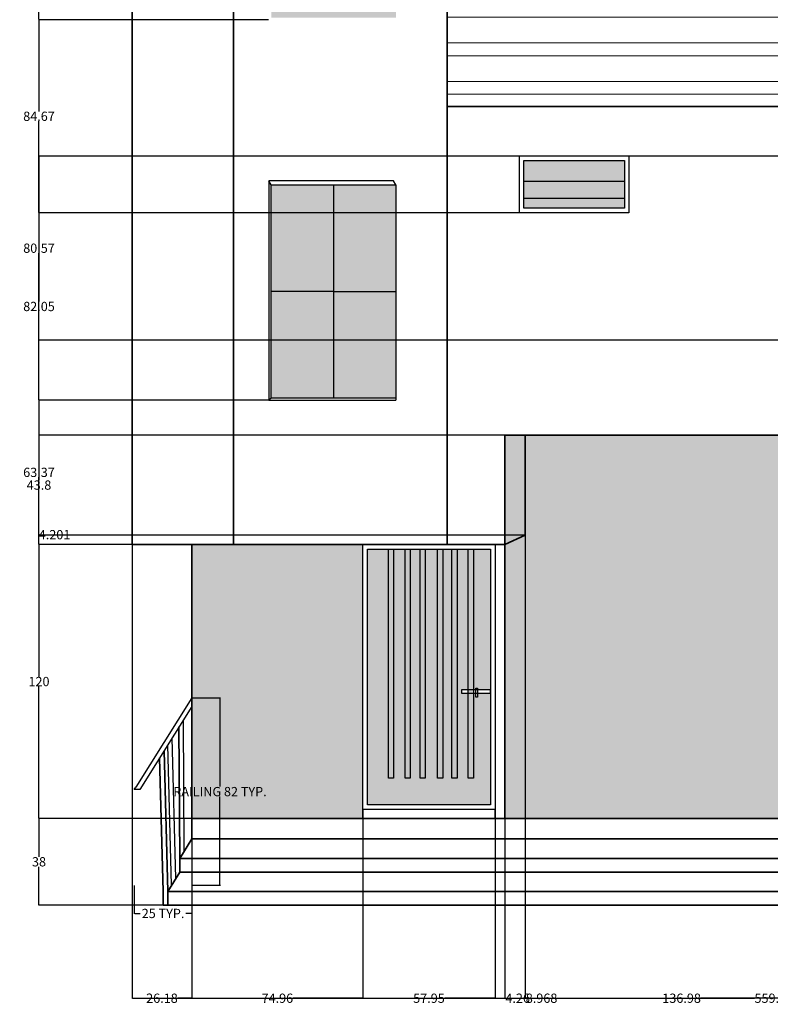
# Model space of a CAD drawing. Units: inches. Extents: x -35 to 623, y 74 to 964.
# Tile 1 of 3: x -35 to 294, y 74 to 505. Entities that reach past the tile are written whole.
import ezdxf

# ---------------------------------------------------------------- set-up
doc = ezdxf.new("R2010")
doc.units = ezdxf.units.IN
doc.header["$MEASUREMENT"] = 0
for name, color, linetype, lineweight in [('A-ANNO-DIMS', 2, 'Continuous', 18), ('A-DOOR', 3, 'Continuous', 25), ('A-ELEV', 7, 'Continuous', 35), ('A-ELEV-PATT', 8, 'Continuous', 13), ('A-FLOR-STRS', 7, 'Continuous', 25), ('A-GLAZ', 4, 'Continuous', 25)]:
    doc.layers.add(name, color=color, linetype=linetype, lineweight=lineweight)
doc.styles.get("Standard").update_dxf_attribs({"font": 'arial.ttf'})
doc.dimstyles.get("Standard").update_dxf_attribs({"dimtxt": 4.0625, "dimasz": 0.18, "dimexe": 0.18, "dimexo": 0.0625, "dimgap": 0.09, "dimtad": 0, "dimtih": 1, "dimtoh": 1, "dimdec": 4, "dimzin": 0, "dimdsep": 46, "dimlunit": 4, "dimtxsty": 'Standard', "dimcen": 0.09, "dimadec": 0, "dimazin": 0, "dimtfac": 1, "dimtdec": 4, "dimtofl": 0, "dimtmove": 0, "dimatfit": 3, "dimfxl": 1, "dimtolj": 1, "dimtzin": 0, "dimarcsym": 0})

# ---------------------------------------------------------------- blocks, each defined once
blk = doc.blocks.new('WIN-TALL-2X2')
for p, q in [((1.05, 94.39), (0, 96.09)), ((0, 96.09), (0, 0)), ((54.58, 96.06), (0, 96.06)), ((55.68, 94.39), (54.58, 96.06)), ((28.36, 94.39), (28.36, 0.82)), ((1.05, 0.82), (0, 0)), ((55.68, 0.82), (55.68, 0)), ((0, 0), (55.68, 0))]:
    blk.add_line(p, q)
blk.add_lwpolyline([(1.05, 94.39), (55.68, 94.39), (55.68, 0.82), (1.05, 0.82)], close=True)
blk = doc.blocks.new('VENT-FRAME')
for points in [[(0, 25.02), (48.03, 25.02), (48.03, 0), (0, 0)], [(2, 23.02), (46.03, 23.02), (46.03, 2), (2, 2)]]:
    blk.add_lwpolyline(points, close=True)
blk = doc.blocks.new('STAIR-RAIL')
for p, q in [((25.22, 82.16), (0.67, 43)), ((25.22, 78.4), (2.36, 41.93)), ((21.93, 15.01), (21.56, 72.56)), ((16.35, 0), (14.7, 61.62)), ((18.27, 3.03), (16.62, 64.68)), ((0, 41.93), (0.67, 43)), ((2.36, 41.93), (0, 41.93))]:
    blk.add_line(p, q)
blk = doc.blocks.new('*D11')
at = {"layer": 'A-ANNO-DIMS', "color": 0, "lineweight": -2, "transparency": 16777216}
for p, q in [((40.51, 207.97), (52.95, 207.97)), ((52.77, 207.79), (52.77, 169.08)), ((52.77, 125.99), (52.77, 164.7)), ((40.51, 125.81), (52.95, 125.81))]:
    blk.add_line(p, q, dxfattribs=at)
at = {"layer": 'A-ANNO-DIMS', "color": 0, "transparency": 16777216}
for points in [[(52.74, 207.79), (52.8, 207.79), (52.77, 207.97)], [(52.74, 125.99), (52.8, 125.99), (52.77, 125.81)]]:
    blk.add_solid(points, dxfattribs=at)
at = {"layer": 'Defpoints', "color": 0, "transparency": 16777216}
for p in [(40.44, 207.97), (52.77, 207.97), (40.44, 125.81)]:
    blk.add_point(p, dxfattribs=at)
at = {"layer": 'A-ANNO-DIMS', "color": 0, "transparency": 16777216, "insert": (52.77, 166.89), "char_height": 4.0625, "attachment_point": 5}
blk.add_mtext('\\A1;RAILING 82 TYP.', dxfattribs=at)
blk = doc.blocks.new('*D12')
at = {"layer": 'A-ANNO-DIMS', "color": 0, "lineweight": -2, "transparency": 16777216}
for p, q in [((15.22, 125.75), (15.22, 113.31)), ((40.44, 125.75), (40.44, 113.31)), ((15.4, 113.49), (17.82, 113.49)), ((40.26, 113.49), (37.84, 113.49))]:
    blk.add_line(p, q, dxfattribs=at)
at = {"layer": 'A-ANNO-DIMS', "color": 0, "transparency": 16777216}
for points in [[(15.4, 113.52), (15.4, 113.46), (15.22, 113.49)], [(40.26, 113.52), (40.26, 113.46), (40.44, 113.49)]]:
    blk.add_solid(points, dxfattribs=at)
at = {"layer": 'Defpoints', "color": 0, "transparency": 16777216}
for p in [(15.22, 125.81), (40.44, 125.81), (40.44, 113.49)]:
    blk.add_point(p, dxfattribs=at)
at = {"layer": 'A-ANNO-DIMS', "color": 0, "transparency": 16777216, "insert": (27.83, 113.49), "char_height": 4.0625, "attachment_point": 5}
blk.add_mtext('\\A1;25 TYP.', dxfattribs=at)
blk = doc.blocks.new('*D13')
at = {"layer": 'A-ANNO-DIMS', "color": 0, "lineweight": -2, "transparency": 16777216}
for p, q in [((14.26, 275.06), (14.26, 76.15)), ((573.64, 167.68), (573.64, 76.15)), ((14.44, 76.33), (287.01, 76.33)), ((573.46, 76.33), (300.89, 76.33))]:
    blk.add_line(p, q, dxfattribs=at)
at = {"layer": 'A-ANNO-DIMS', "color": 0, "transparency": 16777216}
for points in [[(14.44, 76.36), (14.44, 76.3), (14.26, 76.33)], [(573.46, 76.36), (573.46, 76.3), (573.64, 76.33)]]:
    blk.add_solid(points, dxfattribs=at)
at = {"layer": 'Defpoints', "color": 0, "transparency": 16777216}
for p in [(14.26, 275.13), (573.64, 167.74), (573.64, 76.33)]:
    blk.add_point(p, dxfattribs=at)
at = {"layer": 'A-ANNO-DIMS', "color": 0, "transparency": 16777216, "insert": (293.95, 76.33), "char_height": 4.062, "attachment_point": 5}
blk.add_mtext('\\A1;559.4', dxfattribs=at)
blk = doc.blocks.new('*D33')
at = {"layer": 'A-ANNO-DIMS', "color": 0, "lineweight": -2, "transparency": 16777216}
for p, q in [((74.11, 338.49), (-26.72, 338.49)), ((-26.54, 338.31), (-26.54, 308.97)), ((-26.54, 275.31), (-26.54, 304.64)), ((14.2, 275.13), (-26.72, 275.13))]:
    blk.add_line(p, q, dxfattribs=at)
at = {"layer": 'A-ANNO-DIMS', "color": 0, "transparency": 16777216}
for points in [[(-26.57, 338.31), (-26.51, 338.31), (-26.54, 338.49)], [(-26.57, 275.31), (-26.51, 275.31), (-26.54, 275.13)]]:
    blk.add_solid(points, dxfattribs=at)
at = {"layer": 'Defpoints', "color": 0, "transparency": 16777216}
for p in [(-26.54, 338.49), (74.18, 338.49), (14.26, 275.13)]:
    blk.add_point(p, dxfattribs=at)
at = {"layer": 'A-ANNO-DIMS', "color": 0, "transparency": 16777216, "insert": (-26.54, 306.81), "char_height": 4.062, "attachment_point": 5}
blk.add_mtext('\\A1;63.37', dxfattribs=at)
blk = doc.blocks.new('*D34')
at = {"layer": 'A-ANNO-DIMS', "color": 0, "lineweight": -2, "transparency": 16777216}
for p, q in [((183.92, 420.54), (-26.72, 420.54)), ((-26.54, 420.36), (-26.54, 381.68)), ((-26.54, 338.67), (-26.54, 377.35)), ((74.11, 338.49), (-26.72, 338.49))]:
    blk.add_line(p, q, dxfattribs=at)
at = {"layer": 'A-ANNO-DIMS', "color": 0, "transparency": 16777216}
for points in [[(-26.57, 420.36), (-26.51, 420.36), (-26.54, 420.54)], [(-26.57, 338.67), (-26.51, 338.67), (-26.54, 338.49)]]:
    blk.add_solid(points, dxfattribs=at)
at = {"layer": 'Defpoints', "color": 0, "transparency": 16777216}
for p in [(-26.54, 420.54), (183.98, 420.54), (74.18, 338.49)]:
    blk.add_point(p, dxfattribs=at)
at = {"layer": 'A-ANNO-DIMS', "color": 0, "transparency": 16777216, "insert": (-26.54, 379.52), "char_height": 4.062, "attachment_point": 5}
blk.add_mtext('\\A1;82.05', dxfattribs=at)
blk = doc.blocks.new('*D35')
at = {"layer": 'A-ANNO-DIMS', "color": 0, "lineweight": -2, "transparency": 16777216}
for p, q in [((74.11, 505.21), (-26.72, 505.21)), ((-26.54, 505.03), (-26.54, 465.04)), ((-26.54, 420.72), (-26.54, 460.71)), ((183.92, 420.54), (-26.72, 420.54))]:
    blk.add_line(p, q, dxfattribs=at)
at = {"layer": 'A-ANNO-DIMS', "color": 0, "transparency": 16777216}
for points in [[(-26.57, 505.03), (-26.51, 505.03), (-26.54, 505.21)], [(-26.57, 420.72), (-26.51, 420.72), (-26.54, 420.54)]]:
    blk.add_solid(points, dxfattribs=at)
at = {"layer": 'Defpoints', "color": 0, "transparency": 16777216}
for p in [(-26.54, 505.21), (74.18, 505.21), (183.98, 420.54)]:
    blk.add_point(p, dxfattribs=at)
at = {"layer": 'A-ANNO-DIMS', "color": 0, "transparency": 16777216, "insert": (-26.54, 462.88), "char_height": 4.062, "attachment_point": 5}
blk.add_mtext('\\A1;84.67', dxfattribs=at)
blk = doc.blocks.new('*D36')
at = {"layer": 'A-ANNO-DIMS', "color": 0, "lineweight": -2, "transparency": 16777216}
for p, q in [((183.92, 625.8), (-26.72, 625.8)), ((-26.54, 625.62), (-26.54, 567.67)), ((-26.54, 505.39), (-26.54, 563.34)), ((74.11, 505.21), (-26.72, 505.21))]:
    blk.add_line(p, q, dxfattribs=at)
at = {"layer": 'A-ANNO-DIMS', "color": 0, "transparency": 16777216}
for points in [[(-26.57, 625.62), (-26.51, 625.62), (-26.54, 625.8)], [(-26.57, 505.39), (-26.51, 505.39), (-26.54, 505.21)]]:
    blk.add_solid(points, dxfattribs=at)
at = {"layer": 'Defpoints', "color": 0, "transparency": 16777216}
for p in [(-26.54, 625.8), (183.98, 625.8), (74.18, 505.21)]:
    blk.add_point(p, dxfattribs=at)
at = {"layer": 'A-ANNO-DIMS', "color": 0, "transparency": 16777216, "insert": (-26.54, 565.5), "char_height": 4.062, "attachment_point": 5}
blk.add_mtext('\\A1;120.59', dxfattribs=at)
blk = doc.blocks.new('*D42')
at = {"layer": 'A-ANNO-DIMS', "color": 0, "lineweight": -2, "transparency": 16777216}
for p, q in [((14.26, 275.06), (14.26, 76.15)), ((40.44, 155.06), (40.44, 76.15)), ((14.44, 76.33), (20.37, 76.33)), ((40.26, 76.33), (34.34, 76.33))]:
    blk.add_line(p, q, dxfattribs=at)
at = {"layer": 'A-ANNO-DIMS', "color": 0, "transparency": 16777216}
for points in [[(14.44, 76.36), (14.44, 76.3), (14.26, 76.33)], [(40.26, 76.36), (40.26, 76.3), (40.44, 76.33)]]:
    blk.add_solid(points, dxfattribs=at)
at = {"layer": 'Defpoints', "color": 0, "transparency": 16777216}
for p in [(14.26, 275.13), (40.44, 155.13), (40.44, 76.33)]:
    blk.add_point(p, dxfattribs=at)
at = {"layer": 'A-ANNO-DIMS', "color": 0, "transparency": 16777216, "insert": (27.35, 76.33), "char_height": 4.062, "attachment_point": 5}
blk.add_mtext('\\A1;26.18', dxfattribs=at)
blk = doc.blocks.new('*D43')
at = {"layer": 'A-ANNO-DIMS', "color": 0, "lineweight": -2, "transparency": 16777216}
for p, q in [((40.44, 155.06), (40.44, 76.15)), ((115.4, 155.06), (115.4, 76.15)), ((40.62, 76.33), (71, 76.33)), ((115.22, 76.33), (84.85, 76.33))]:
    blk.add_line(p, q, dxfattribs=at)
at = {"layer": 'A-ANNO-DIMS', "color": 0, "transparency": 16777216}
for points in [[(40.62, 76.36), (40.62, 76.3), (40.44, 76.33)], [(115.22, 76.36), (115.22, 76.3), (115.4, 76.33)]]:
    blk.add_solid(points, dxfattribs=at)
at = {"layer": 'Defpoints', "color": 0, "transparency": 16777216}
for p in [(40.44, 155.13), (115.4, 155.13), (115.4, 76.33)]:
    blk.add_point(p, dxfattribs=at)
at = {"layer": 'A-ANNO-DIMS', "color": 0, "transparency": 16777216, "insert": (77.92, 76.33), "char_height": 4.062, "attachment_point": 5}
blk.add_mtext('\\A1;74.96', dxfattribs=at)
blk = doc.blocks.new('*D44')
at = {"layer": 'A-ANNO-DIMS', "color": 0, "lineweight": -2, "transparency": 16777216}
for p, q in [((115.4, 155.06), (115.4, 76.15)), ((173.35, 155.06), (173.35, 76.15)), ((115.58, 76.33), (137.42, 76.33)), ((173.17, 76.33), (151.33, 76.33))]:
    blk.add_line(p, q, dxfattribs=at)
at = {"layer": 'A-ANNO-DIMS', "color": 0, "transparency": 16777216}
for points in [[(115.58, 76.36), (115.58, 76.3), (115.4, 76.33)], [(173.17, 76.36), (173.17, 76.3), (173.35, 76.33)]]:
    blk.add_solid(points, dxfattribs=at)
at = {"layer": 'Defpoints', "color": 0, "transparency": 16777216}
for p in [(115.4, 155.13), (173.35, 155.13), (173.35, 76.33)]:
    blk.add_point(p, dxfattribs=at)
at = {"layer": 'A-ANNO-DIMS', "color": 0, "transparency": 16777216, "insert": (144.37, 76.33), "char_height": 4.062, "attachment_point": 5}
blk.add_mtext('\\A1;57.95', dxfattribs=at)
blk = doc.blocks.new('*D45')
at = {"layer": 'A-ANNO-DIMS', "color": 0, "lineweight": -2, "transparency": 16777216}
for p, q in [((173.35, 155.06), (173.35, 76.15)), ((177.61, 155.06), (177.61, 76.15)), ((173.53, 76.33), (177.43, 76.33)), ((177.61, 76.33), (177.79, 76.33))]:
    blk.add_line(p, q, dxfattribs=at)
at = {"layer": 'A-ANNO-DIMS', "color": 0, "transparency": 16777216}
for points in [[(173.53, 76.36), (173.53, 76.3), (173.35, 76.33)], [(177.43, 76.36), (177.43, 76.3), (177.61, 76.33)]]:
    blk.add_solid(points, dxfattribs=at)
at = {"layer": 'Defpoints', "color": 0, "transparency": 16777216}
for p in [(173.35, 155.13), (177.61, 155.13), (177.61, 76.33)]:
    blk.add_point(p, dxfattribs=at)
at = {"layer": 'A-ANNO-DIMS', "color": 0, "transparency": 16777216, "insert": (183.24, 76.33), "char_height": 4.062, "attachment_point": 5}
blk.add_mtext('\\A1;4.26', dxfattribs=at)
blk = doc.blocks.new('*D46')
at = {"layer": 'A-ANNO-DIMS', "color": 0, "lineweight": -2, "transparency": 16777216}
for p, q in [((186.58, 279.26), (186.58, 76.15)), ((177.61, 155.06), (177.61, 76.15)), ((177.79, 76.33), (186.4, 76.33)), ((186.58, 76.33), (186.76, 76.33))]:
    blk.add_line(p, q, dxfattribs=at)
at = {"layer": 'A-ANNO-DIMS', "color": 0, "transparency": 16777216}
for points in [[(177.79, 76.36), (177.79, 76.3), (177.61, 76.33)], [(186.4, 76.36), (186.4, 76.3), (186.58, 76.33)]]:
    blk.add_solid(points, dxfattribs=at)
at = {"layer": 'Defpoints', "color": 0, "transparency": 16777216}
for p in [(186.58, 279.33), (177.61, 155.13), (186.58, 76.33)]:
    blk.add_point(p, dxfattribs=at)
at = {"layer": 'A-ANNO-DIMS', "color": 0, "transparency": 16777216, "insert": (193.71, 76.33), "char_height": 4.062, "attachment_point": 5}
blk.add_mtext('\\A1;8.968', dxfattribs=at)
blk = doc.blocks.new('*D47')
at = {"layer": 'A-ANNO-DIMS', "color": 0, "lineweight": -2, "transparency": 16777216}
for p, q in [((186.58, 279.26), (186.58, 76.15)), ((323.56, 155.06), (323.56, 76.15)), ((186.76, 76.33), (246.74, 76.33)), ((323.38, 76.33), (263.41, 76.33))]:
    blk.add_line(p, q, dxfattribs=at)
at = {"layer": 'A-ANNO-DIMS', "color": 0, "transparency": 16777216}
for points in [[(186.76, 76.36), (186.76, 76.3), (186.58, 76.33)], [(323.38, 76.36), (323.38, 76.3), (323.56, 76.33)]]:
    blk.add_solid(points, dxfattribs=at)
at = {"layer": 'Defpoints', "color": 0, "transparency": 16777216}
for p in [(186.58, 279.33), (323.56, 155.13), (323.56, 76.33)]:
    blk.add_point(p, dxfattribs=at)
at = {"layer": 'A-ANNO-DIMS', "color": 0, "transparency": 16777216, "insert": (255.07, 76.33), "char_height": 4.062, "attachment_point": 5}
blk.add_mtext('\\A1;136.98', dxfattribs=at)
blk = doc.blocks.new('*D54')
at = {"layer": 'A-ANNO-DIMS', "color": 0, "lineweight": -2, "transparency": 16777216}
for p, q in [((40.38, 155.13), (-26.72, 155.13)), ((-26.54, 154.95), (-26.54, 138.29)), ((-26.54, 117.31), (-26.54, 133.96)), ((29.84, 117.13), (-26.72, 117.13))]:
    blk.add_line(p, q, dxfattribs=at)
at = {"layer": 'A-ANNO-DIMS', "color": 0, "transparency": 16777216}
for points in [[(-26.57, 154.95), (-26.51, 154.95), (-26.54, 155.13)], [(-26.57, 117.31), (-26.51, 117.31), (-26.54, 117.13)]]:
    blk.add_solid(points, dxfattribs=at)
at = {"layer": 'Defpoints', "color": 0, "transparency": 16777216}
for p in [(-26.54, 155.13), (40.44, 155.13), (29.91, 117.13)]:
    blk.add_point(p, dxfattribs=at)
at = {"layer": 'A-ANNO-DIMS', "color": 0, "transparency": 16777216, "insert": (-26.54, 136.13), "char_height": 4.062, "attachment_point": 5}
blk.add_mtext('\\A1;38', dxfattribs=at)
blk = doc.blocks.new('*D55')
at = {"layer": 'A-ANNO-DIMS', "color": 0, "lineweight": -2, "transparency": 16777216}
for p, q in [((14.2, 275.13), (-26.72, 275.13)), ((-26.54, 274.95), (-26.54, 217.29)), ((-26.54, 155.31), (-26.54, 212.96)), ((40.38, 155.13), (-26.72, 155.13))]:
    blk.add_line(p, q, dxfattribs=at)
at = {"layer": 'A-ANNO-DIMS', "color": 0, "transparency": 16777216}
for points in [[(-26.57, 274.95), (-26.51, 274.95), (-26.54, 275.13)], [(-26.57, 155.31), (-26.51, 155.31), (-26.54, 155.13)]]:
    blk.add_solid(points, dxfattribs=at)
at = {"layer": 'Defpoints', "color": 0, "transparency": 16777216}
for p in [(-26.54, 275.13), (14.26, 275.13), (40.44, 155.13)]:
    blk.add_point(p, dxfattribs=at)
at = {"layer": 'A-ANNO-DIMS', "color": 0, "transparency": 16777216, "insert": (-26.54, 215.13), "char_height": 4.062, "attachment_point": 5}
blk.add_mtext('\\A1;120', dxfattribs=at)
blk = doc.blocks.new('*D56')
at = {"layer": 'A-ANNO-DIMS', "color": 0, "lineweight": -2, "transparency": 16777216}
for p, q in [((186.52, 279.33), (-26.72, 279.33)), ((-26.54, 279.33), (-26.54, 279.51)), ((-26.54, 279.51), (-26.36, 279.51)), ((-26.54, 275.31), (-26.54, 279.15)), ((14.2, 275.13), (-26.72, 275.13))]:
    blk.add_line(p, q, dxfattribs=at)
at = {"layer": 'A-ANNO-DIMS', "color": 0, "transparency": 16777216}
for points in [[(-26.57, 279.15), (-26.51, 279.15), (-26.54, 279.33)], [(-26.57, 275.31), (-26.51, 275.31), (-26.54, 275.13)]]:
    blk.add_solid(points, dxfattribs=at)
at = {"layer": 'Defpoints', "color": 0, "transparency": 16777216}
for p in [(-26.54, 279.33), (186.58, 279.33), (14.26, 275.13)]:
    blk.add_point(p, dxfattribs=at)
at = {"layer": 'A-ANNO-DIMS', "color": 0, "transparency": 16777216, "insert": (-19.72, 279.51), "char_height": 4.062, "attachment_point": 5}
blk.add_mtext('\\A1;4.201', dxfattribs=at)
blk = doc.blocks.new('*D57')
at = {"layer": 'A-ANNO-DIMS', "color": 0, "lineweight": -2, "transparency": 16777216}
for p, q in [((186.52, 323.13), (-26.72, 323.13)), ((-26.54, 322.95), (-26.54, 303.39)), ((-26.54, 279.51), (-26.54, 299.06)), ((186.52, 279.33), (-26.72, 279.33))]:
    blk.add_line(p, q, dxfattribs=at)
at = {"layer": 'A-ANNO-DIMS', "color": 0, "transparency": 16777216}
for points in [[(-26.57, 322.95), (-26.51, 322.95), (-26.54, 323.13)], [(-26.57, 279.51), (-26.51, 279.51), (-26.54, 279.33)]]:
    blk.add_solid(points, dxfattribs=at)
at = {"layer": 'Defpoints', "color": 0, "transparency": 16777216}
for p in [(-26.54, 323.13), (186.58, 323.13), (186.58, 279.33)]:
    blk.add_point(p, dxfattribs=at)
at = {"layer": 'A-ANNO-DIMS', "color": 0, "transparency": 16777216, "insert": (-26.54, 301.23), "char_height": 4.062, "attachment_point": 5}
blk.add_mtext('\\A1;43.8', dxfattribs=at)
blk = doc.blocks.new('*D74')
at = {"layer": 'A-ANNO-DIMS', "color": 0, "lineweight": -2, "transparency": 16777216}
for p, q in [((359.73, 445.34), (-26.72, 445.34)), ((-26.54, 445.16), (-26.54, 407.23)), ((-26.54, 364.96), (-26.54, 402.9)), ((359.73, 364.78), (-26.72, 364.78))]:
    blk.add_line(p, q, dxfattribs=at)
at = {"layer": 'A-ANNO-DIMS', "color": 0, "transparency": 16777216}
for points in [[(-26.57, 445.16), (-26.51, 445.16), (-26.54, 445.34)], [(-26.57, 364.96), (-26.51, 364.96), (-26.54, 364.78)]]:
    blk.add_solid(points, dxfattribs=at)
at = {"layer": 'Defpoints', "color": 0, "transparency": 16777216}
for p in [(-26.54, 445.34), (359.79, 445.34), (359.79, 364.78)]:
    blk.add_point(p, dxfattribs=at)
at = {"layer": 'A-ANNO-DIMS', "color": 0, "transparency": 16777216, "insert": (-26.54, 405.06), "char_height": 4.062, "attachment_point": 5}
blk.add_mtext('\\A1;80.57', dxfattribs=at)

msp = doc.modelspace()

# ---------------------------------------------------------------- hatches: boundary and pattern name
at = {"layer": 'A-ELEV-PATT'}
h = msp.add_hatch(color=256, dxfattribs=at)
h.dxf.hatch_style = 1
h.set_gradient(color2=(99, 100, 102))
h.paths.add_polyline_path([(471.0064, 631.4927), (434.7868, 631.4927), (434.7868, 579.8536), (471.0064, 579.8536)])
h.paths.add_polyline_path([(509.226, 631.4927), (473.0064, 631.4927), (473.0064, 579.8536), (509.226, 579.8536)])
h.paths.add_polyline_path([(449.3739, 427.1438), (413.1543, 427.1438), (413.1543, 380.7902), (449.3739, 380.7902)])
h.paths.add_polyline_path([(411.1543, 427.1438), (374.9347, 427.1438), (374.9347, 380.7902), (411.1543, 380.7902)])
h.paths.add_polyline_path([(374.9294, 263.937), (338.7098, 263.937), (338.7098, 217.5834), (374.9294, 217.5834)])
h.paths.add_polyline_path([(413.1491, 263.937), (376.9294, 263.937), (376.9294, 217.5834), (413.1491, 217.5834)])
h.paths.add_polyline_path([(230.0086, 434.3669), (185.9817, 434.3669), (185.9817, 426.9441), (230.0086, 426.9441)])
h.paths.add_polyline_path([(230.0086, 443.5602), (185.9817, 443.5602), (185.9817, 434.3669), (230.0086, 434.3669)])
h.paths.add_polyline_path([(230.0086, 426.9441), (185.9817, 426.9441), (185.9817, 422.542), (230.0086, 422.542)])
h.paths.add_polyline_path([(230.0086, 648.8148), (185.9817, 648.8148), (185.9817, 642.5298), (230.0086, 642.5298)])
h.paths.add_polyline_path([(230.0086, 642.5298), (185.9817, 642.5298), (185.9817, 633.9381), (230.0086, 633.9381)])
h.paths.add_polyline_path([(230.0086, 633.9381), (185.9817, 633.9381), (185.9817, 627.7966), (230.0086, 627.7966)])
h.paths.add_polyline_path([(230.0086, 863.7512), (185.9817, 863.7512), (185.9817, 856.0022), (230.0086, 856.0022)])
h.paths.add_polyline_path([(230.0086, 856.0022), (185.9817, 856.0022), (185.9817, 849.1652), (230.0086, 849.1652)])
h.paths.add_polyline_path([(230.0086, 849.1652), (185.9817, 849.1652), (185.9817, 842.733), (230.0086, 842.733)])
h = msp.add_hatch(dxfattribs=at)
h.set_pattern_fill('ANSI32', color=256, scale=45, angle=135)
h.paths.add_polyline_path([(548.4175, 755.1261), (152.2908, 755.1261), (152.2908, 611.1261), (152.2908, 467.1261), (548.4175, 467.1261), (548.4175, 544.5164), (425.7698, 544.5164), (425.7698, 649.844), (548.4175, 649.844)])
h.paths.add_polyline_path([(232.0086, 650.8148), (232.0086, 625.7966), (183.9817, 625.7966), (183.9817, 650.8148)], flags=16)
h.paths.add_polyline_path([(230.0086, 648.8148), (230.0086, 627.7966), (185.9817, 627.7966), (185.9817, 648.8148)], flags=0)
h = msp.add_hatch(color=256, dxfattribs=at)
h.dxf.hatch_style = 1
h.set_gradient(color2=(99, 100, 102))
h.paths.add_polyline_path([(129.855, 386.1003), (102.5419, 386.1003), (102.5419, 339.3154), (129.855, 339.3154)])
h.paths.add_polyline_path([(129.855, 432.8853), (102.5419, 432.8853), (102.5419, 386.1003), (129.855, 386.1003)])
h.paths.add_polyline_path([(102.5419, 432.8853), (75.2288, 432.8853), (75.2288, 386.1003), (102.5419, 386.1003)])
h.paths.add_polyline_path([(102.5419, 386.1003), (75.2288, 386.1003), (75.2288, 339.3154), (102.5419, 339.3154)])
h.paths.add_polyline_path([(102.5419, 599.6034), (75.2288, 599.6034), (75.2288, 552.8184), (102.5419, 552.8184)])
h.paths.add_polyline_path([(129.855, 599.6034), (102.5419, 599.6034), (102.5419, 552.8184), (129.855, 552.8184)])
h.paths.add_polyline_path([(129.855, 552.8184), (102.5419, 552.8184), (102.5419, 506.0335), (129.855, 506.0335)])
h.paths.add_polyline_path([(102.5419, 552.8184), (75.2288, 552.8184), (75.2288, 506.0335), (102.5419, 506.0335)])
h = msp.add_hatch(color=256, dxfattribs=at)
h.dxf.hatch_style = 1
h.set_gradient(color1=(199, 200, 202), color2=(99, 100, 102))
h.paths.add_polyline_path([(323.5636, 282.1377), (323.5636, 323.1261), (186.5792, 323.1261), (186.5792, 279.3267), (177.6113, 275.1261), (177.6113, 155.1261), (323.5636, 155.1261), (323.5636, 201.572)])
h.paths.add_polyline_path([(548.4175, 323.1261), (429.1717, 323.1261), (429.1717, 282.1377), (429.1717, 201.572), (429.1717, 155.1261), (548.4175, 155.1261)])
h.paths.add_polyline_path([(115.3998, 275.1261), (40.4435, 275.1261), (40.4435, 155.1261), (115.3998, 155.1261), (115.3998, 159.0807)])
h.paths.add_polyline_path([(126.5574, 273.1261), (117.3998, 273.1261), (117.3998, 161.0807), (171.3498, 161.0807), (171.3498, 210.0445), (165.6209, 210.0445), (165.6209, 208.3223), (164.9007, 208.3223), (164.9007, 210.0445), (163.8747, 210.0445), (163.8747, 172.7632), (161.5924, 172.7632), (161.5924, 210.0445), (158.6465, 210.0445), (158.6465, 211.5523), (161.5924, 211.5523), (161.5924, 273.1261), (156.6973, 273.1261), (156.6973, 172.7632), (154.4151, 172.7632), (154.4151, 273.1261), (150.4171, 273.1261), (150.4171, 172.7632), (148.1349, 172.7632), (148.1349, 273.1261), (142.7413, 273.1261), (142.7413, 172.7632), (140.4591, 172.7632), (140.4591, 273.1261), (136.1621, 273.1261), (136.1621, 172.7632), (133.8798, 172.7632), (133.8798, 273.1261), (128.8396, 273.1261), (128.8396, 172.7632), (126.5574, 172.7632)])
h.paths.add_polyline_path([(171.3498, 273.1261), (163.8747, 273.1261), (163.8747, 211.5523), (164.9007, 211.5523), (164.9007, 212.2403), (165.6209, 212.2403), (165.6209, 211.5523), (171.3498, 211.5523)], flags=17)
h.paths.add_polyline_path([(186.5792, 323.1261), (177.6113, 323.1261), (177.6113, 275.1261), (186.5792, 279.3267)], flags=17)
h = msp.add_hatch(color=256, dxfattribs=at)
h.dxf.hatch_style = 1
h.paths.add_polyline_path([(128.8396, 273.1261), (126.5574, 273.1261), (126.5574, 172.7632), (128.8396, 172.7632)])
h.paths.add_polyline_path([(136.1621, 273.1261), (133.8798, 273.1261), (133.8798, 172.7632), (136.1621, 172.7632)])
h.paths.add_polyline_path([(142.7413, 273.1261), (140.4591, 273.1261), (140.4591, 172.7632), (142.7413, 172.7632)])
h.paths.add_polyline_path([(150.4171, 273.1261), (148.1349, 273.1261), (148.1349, 172.7632), (150.4171, 172.7632)])
h.paths.add_polyline_path([(156.6973, 273.1261), (154.4151, 273.1261), (154.4151, 172.7632), (156.6973, 172.7632)])
h = msp.add_hatch(color=256, dxfattribs=at)
h.dxf.hatch_style = 1
h.paths.add_polyline_path([(163.8747, 273.1261), (161.5924, 273.1261), (161.5924, 211.5523), (163.8747, 211.5523)])
h.paths.add_polyline_path([(163.8747, 210.0445), (161.5924, 210.0445), (161.5924, 172.7632), (163.8747, 172.7632)])
h.paths.add_polyline_path([(163.8747, 211.5523), (161.5924, 211.5523), (161.5924, 210.0445), (163.8747, 210.0445)])

# ---------------------------------------------------------------- linework, layer by layer
at = {"layer": 'A-DOOR'}
for points in [[(115.3998, 275.1261), (173.3498, 275.1261), (173.3498, 159.0807), (115.3998, 159.0807)], [(117.3998, 273.1261), (171.3498, 273.1261), (171.3498, 161.0807), (117.3998, 161.0807)], [(126.5574, 273.1261), (128.8396, 273.1261), (128.8396, 172.7632), (126.5574, 172.7632)], [(133.8798, 273.1261), (136.1621, 273.1261), (136.1621, 172.7632), (133.8798, 172.7632)], [(140.4591, 273.1261), (142.7413, 273.1261), (142.7413, 172.7632), (140.4591, 172.7632)], [(148.1349, 273.1261), (150.4171, 273.1261), (150.4171, 172.7632), (148.1349, 172.7632)], [(154.4151, 273.1261), (156.6973, 273.1261), (156.6973, 172.7632), (154.4151, 172.7632)], [(161.5924, 273.1261), (163.8747, 273.1261), (163.8747, 172.7632), (161.5924, 172.7632)], [(171.3498, 211.5523), (158.6465, 211.5523), (158.6465, 210.0445), (171.3498, 210.0445)], [(164.9007, 212.2403), (165.6209, 212.2403), (165.6209, 208.3223), (164.9007, 208.3223)]]:
    msp.add_lwpolyline(points, close=True, dxfattribs=at)
at = {"layer": 'A-ELEV'}
for p, q in [((14.262, 467.2972), (14.262, 611.2972)), ((58.6458, 467.1261), (58.6458, 611.1261)), ((152.2908, 467.1261), (152.2908, 611.1261)), ((14.262, 275.1261), (14.262, 467.2972)), ((58.6458, 275.1261), (58.6458, 467.1261)), ((152.2908, 467.1261), (548.4175, 467.1261)), ((152.2908, 275.1261), (152.2908, 467.1261)), ((548.4175, 323.1261), (177.6113, 323.1261)), ((177.6113, 323.1261), (177.6113, 155.1261)), ((177.6113, 323.1261), (177.6113, 275.1261)), ((186.5792, 279.3267), (186.5792, 323.1261)), ((177.6113, 275.1261), (186.5792, 279.3267)), ((40.4435, 275.1261), (14.262, 275.1261)), ((177.6113, 275.1261), (40.4435, 275.1261)), ((40.4435, 275.1261), (40.4435, 155.1261)), ((35.175, 137.6266), (34.8026, 195.2104)), ((27.9071, 123.0737), (26.3428, 181.7174)), ((29.9064, 123.127), (28.2618, 184.7782)), ((115.3998, 159.0807), (115.3998, 159.0807)), ((115.3998, 159.0807), (115.3998, 155.1261)), ((173.3498, 159.0807), (173.3498, 155.1261)), ((40.4435, 155.1261), (548.4175, 155.1261)), ((40.4435, 155.1261), (40.4435, 146.1261)), ((40.4435, 146.1261), (35.175, 137.6266)), ((40.4435, 146.1261), (548.4175, 146.1261)), ((35.175, 137.6266), (553.6861, 137.6266)), ((35.175, 137.6266), (35.175, 131.6266)), ((35.175, 131.6266), (29.9064, 123.127)), ((35.175, 131.6266), (553.6861, 131.6266)), ((27.9071, 123.0737), (27.9071, 117.127)), ((29.9064, 123.127), (558.9547, 123.127)), ((29.9064, 117.127), (29.9064, 123.127)), ((27.9071, 117.127), (29.9064, 117.127)), ((558.9547, 117.127), (29.9064, 117.127))]:
    msp.add_line(p, q, dxfattribs=at)
at = {"layer": 'A-GLAZ'}
for p, q in [((185.9817, 434.3669), (230.0086, 434.3669)), ((185.9817, 426.9441), (230.0086, 426.9441)), ((102.5419, 386.1003), (75.2288, 386.1003)), ((102.5419, 386.1003), (129.855, 386.1003))]:
    msp.add_line(p, q, dxfattribs=at)

# ---------------------------------------------------------------- block references
at = {"layer": 'A-FLOR-STRS'}
msp.add_blockref('STAIR-RAIL', (15.221, 125.81), dxfattribs=at)
at = {"layer": 'A-GLAZ'}
for name, p in [('VENT-FRAME', (183.982, 420.542)), ('WIN-TALL-2X2', (74.177, 338.4928))]:
    msp.add_blockref(name, p, dxfattribs=at)

# ---------------------------------------------------------------- dimensions: what is measured, and where the dimension line sits
at = {"layer": 'A-ANNO-DIMS'}
for base, p1, p2, override, picture, middle in [((-26.538, 625.7966), (74.1775, 505.2106), (183.9817, 625.7966), {"dimdec": 2, "dimlfac": 1, "dimrnd": 0, "dimzin": 0, "dimdsep": 46, "dimlunit": 2}, '*D36', (-26.538, 565.5036)), ((-26.538, 505.2106), (183.9817, 420.542), (74.1775, 505.2106), {"dimdec": 2, "dimlfac": 1, "dimrnd": 0, "dimzin": 0, "dimdsep": 46, "dimlunit": 2}, '*D35', (-26.538, 462.8763)), ((-26.538, 445.3445), (359.7884, 364.7788), (359.7884, 445.3445), {"dimdec": 2, "dimlfac": 1, "dimrnd": 0, "dimzin": 0, "dimdsep": 46, "dimlunit": 2}, '*D74', (-26.538, 405.0617)), ((-26.538, 420.542), (74.1775, 338.4925), (183.9817, 420.542), {"dimdec": 2, "dimlfac": 1, "dimrnd": 0, "dimzin": 0, "dimdsep": 46, "dimlunit": 2}, '*D34', (-26.538, 379.5172)), ((-26.538, 338.4925), (14.262, 275.1261), (74.1775, 338.4925), {"dimdec": 2, "dimlfac": 1, "dimrnd": 0, "dimzin": 0, "dimdsep": 46, "dimlunit": 2}, '*D33', (-26.538, 306.8093)), ((-26.538, 323.1261), (186.5792, 279.3267), (186.5792, 323.1261), {"dimdec": 1, "dimlfac": 1, "dimrnd": 0, "dimzin": 0, "dimdsep": 46, "dimlunit": 2}, '*D57', (-26.538, 301.2264)), ((-26.538, 279.3267), (14.262, 275.1261), (186.5792, 279.3267), {"dimdec": 3, "dimlfac": 1, "dimrnd": 0, "dimzin": 0, "dimdsep": 46, "dimlunit": 2}, '*D56', (-19.7239, 279.5067)), ((-26.538, 275.1261), (40.4435, 155.1261), (14.262, 275.1261), {"dimdec": 0, "dimlfac": 1, "dimrnd": 0, "dimzin": 0, "dimdsep": 46, "dimlunit": 2}, '*D55', (-26.538, 215.1261)), ((-26.538, 155.1261), (29.9064, 117.127), (40.4435, 155.1261), {"dimdec": 0, "dimlfac": 1, "dimrnd": 0, "dimzin": 0, "dimdsep": 46, "dimlunit": 2}, '*D54', (-26.538, 136.1266))]:
    dim = msp.add_linear_dim(base=base, p1=p1, p2=p2, angle=90, dimstyle='Standard', override=override, dxfattribs=at)
    dim.commit()
    dim.dimension.update_dxf_attribs({"geometry": picture, "text_midpoint": middle})
for base, p1, p2, override, picture, middle in [((186.5792, 76.327), (177.6113, 155.1261), (186.5792, 279.3267), {"dimdec": 3, "dimlfac": 1, "dimrnd": 0, "dimzin": 0, "dimdsep": 46, "dimlunit": 2}, '*D46', (193.7106, 76.327)), ((323.5636, 76.327), (186.5792, 279.3267), (323.5636, 155.1261), {"dimdec": 2, "dimlfac": 1, "dimrnd": 0, "dimzin": 0, "dimdsep": 46, "dimlunit": 2}, '*D47', (255.0714, 76.327)), ((573.6397, 76.327), (14.262, 275.1261), (573.6397, 167.7443), {"dimdec": 1, "dimlfac": 1, "dimrnd": 0, "dimzin": 0, "dimdsep": 46, "dimlunit": 2}, '*D13', (293.9509, 76.327)), ((40.4435, 76.327), (14.262, 275.1261), (40.4435, 155.1261), {"dimdec": 2, "dimlfac": 1, "dimrnd": 0, "dimzin": 0, "dimdsep": 46, "dimlunit": 2}, '*D42', (27.3528, 76.327)), ((115.3998, 76.327), (40.4435, 155.1261), (115.3998, 155.1261), {"dimdec": 2, "dimlfac": 1, "dimrnd": 0, "dimzin": 0, "dimdsep": 46, "dimlunit": 2}, '*D43', (77.9217, 76.327)), ((173.3498, 76.327), (115.3998, 155.1261), (173.3498, 155.1261), {"dimdec": 2, "dimlfac": 1, "dimrnd": 0, "dimzin": 0, "dimdsep": 46, "dimlunit": 2}, '*D44', (144.3748, 76.327)), ((177.6113, 76.327), (173.3498, 155.1261), (177.6113, 155.1261), {"dimdec": 2, "dimlfac": 1, "dimrnd": 0, "dimzin": 0, "dimdsep": 46, "dimlunit": 2}, '*D45', (183.2379, 76.327))]:
    dim = msp.add_linear_dim(base=base, p1=p1, p2=p2, dimstyle='Standard', override=override, dxfattribs=at)
    dim.commit()
    dim.dimension.update_dxf_attribs({"geometry": picture, "text_midpoint": middle})
dim = msp.add_linear_dim(base=(52.7679, 207.9725), p1=(40.4435, 125.8103), p2=(40.4435, 207.9725), angle=90, text='RAILING <> TYP.', dimstyle='Standard', override={"dimdec": 0, "dimlfac": 1, "dimrnd": 0, "dimzin": 0, "dimdsep": 46, "dimlunit": 2}, dxfattribs=at)
dim.commit()
dim.dimension.update_dxf_attribs({"geometry": '*D11', "text_midpoint": (52.7679, 166.8914)})
dim = msp.add_linear_dim(base=(40.4435, 113.4859), p1=(15.2213, 125.8103), p2=(40.4435, 125.8103), text='<> TYP.', dimstyle='Standard', override={"dimdec": 0, "dimlfac": 1, "dimrnd": 0, "dimzin": 0, "dimdsep": 46, "dimlunit": 2}, dxfattribs=at)
dim.commit()
dim.dimension.update_dxf_attribs({"geometry": '*D12', "text_midpoint": (27.8324, 113.4859)})

doc.saveas('drawing.dxf')
